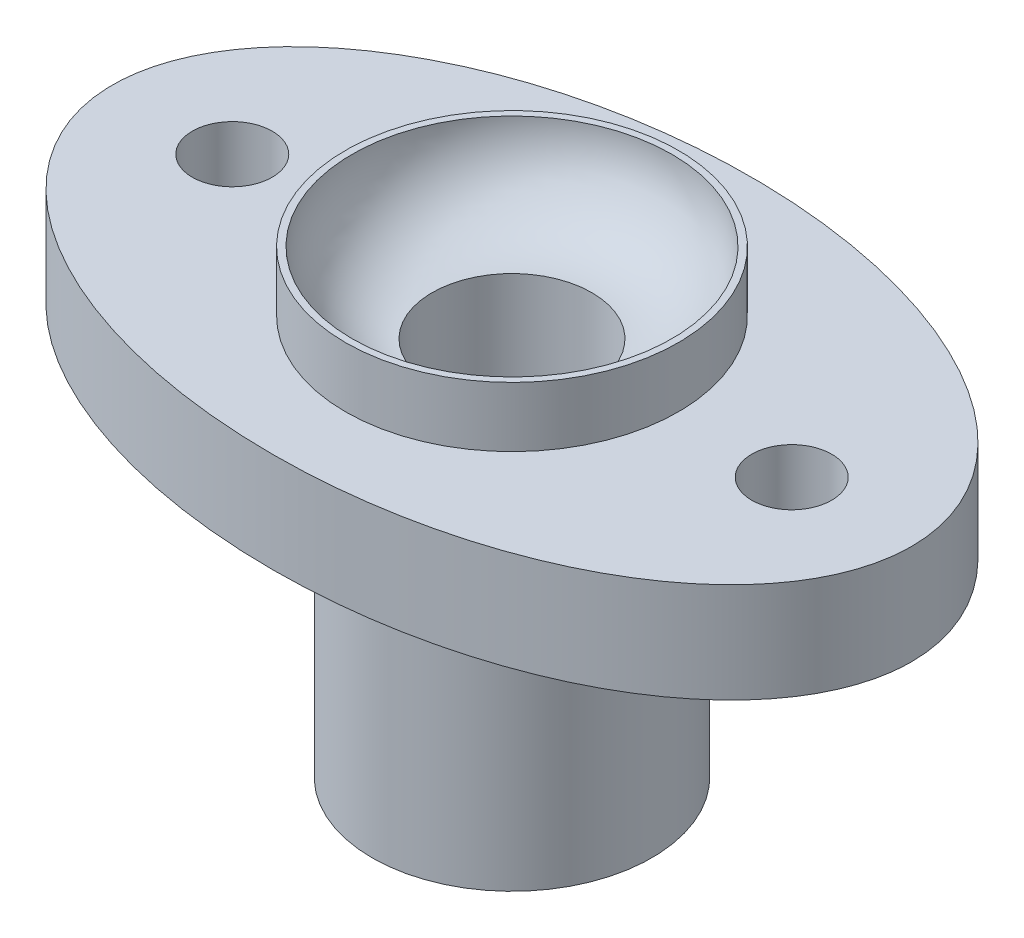
from build123d import *

# Parameters (mm, degrees)
SHANK_SKETCH_42_R          = 21
SHANK_42_DEPTH             = 45
FLANGE_SKETCH_120X36_RX    = 60
FLANGE_SKETCH_120X36_RY    = 36
OVAL_FLANGE_120X36_DEPTH   = 15
SPIGOT_SKETCH_50_R         = 25
SPIGOT_50_DEPTH            = 9
MOUNTING_HOLES_SKETCH_R    = 6
MOUNTING_HOLES_2X_12_DEPTH = 19


with BuildPart() as part:
    # Shank Sketch Ø42 → Shank Ø42 (new body)
    with BuildSketch(Plane(origin=(0, 0, 0), x_dir=(1, 0, 0), z_dir=(0, 1, 0))):
        with Locations(Location((0, 0, 0), (0, 0, 90))):
            Circle(SHANK_SKETCH_42_R)
    extrude(amount=SHANK_42_DEPTH)

    # Flange Sketch 120x36 → Oval Flange 120x36 (add)
    with BuildSketch(Plane(origin=(0, 45, 0), x_dir=(1, 0, 0), z_dir=(0, 1, 0))):
        with Locations((0, 0)):
            Ellipse(FLANGE_SKETCH_120X36_RX, FLANGE_SKETCH_120X36_RY)
    extrude(amount=OVAL_FLANGE_120X36_DEPTH)

    # Spigot Sketch Ø50 → Spigot Ø50 (add)
    with BuildSketch(Plane(origin=(0, 60, 0), x_dir=(1, 0, 0), z_dir=(0, 1, 0))):
        with Locations(Location((0, 0, 0), (0, 0, 270))):
            Circle(SPIGOT_SKETCH_50_R)
    extrude(amount=SPIGOT_50_DEPTH)

    # Bore Profile Sketch → Bore and Seat Cut (revolve, cut)
    with BuildSketch(Plane.XY, mode=Mode.PRIVATE) as bore_and_seat_cut_sk:
        with BuildLine():
            Line((21, 0), (12, 2.411542732))
            Line((12, 2.411542732), (12, 57))
            ThreePointArc((12, 57), (20.485281374, 60.514718626), (24, 69))
            Line((24, 69), (0, 69))
            Line((0, 69), (0, 0))
            Line((0, 0), (21, 0))
        make_face()
    revolve(bore_and_seat_cut_sk.sketch.rotate(Axis((0, 0, 0), (0, 1, 0)), 90), axis=Axis((0, 0, 0), (0, 1, 0)), mode=Mode.SUBTRACT)

    # Mounting Holes Sketch → Mounting Holes 2xØ12 (cut)
    with BuildSketch(Plane(origin=(0, 60, 0), x_dir=(1, 0, 0), z_dir=(0, 1, 0))):
        with Locations(Location((-42, 0, 0), (0, 0, 270))):
            Circle(MOUNTING_HOLES_SKETCH_R)
        with Locations(Location((42, 0, 0), (0, 0, 270))):
            Circle(MOUNTING_HOLES_SKETCH_R)
    extrude(amount=-MOUNTING_HOLES_2X_12_DEPTH, mode=Mode.SUBTRACT)


solid = part.part
